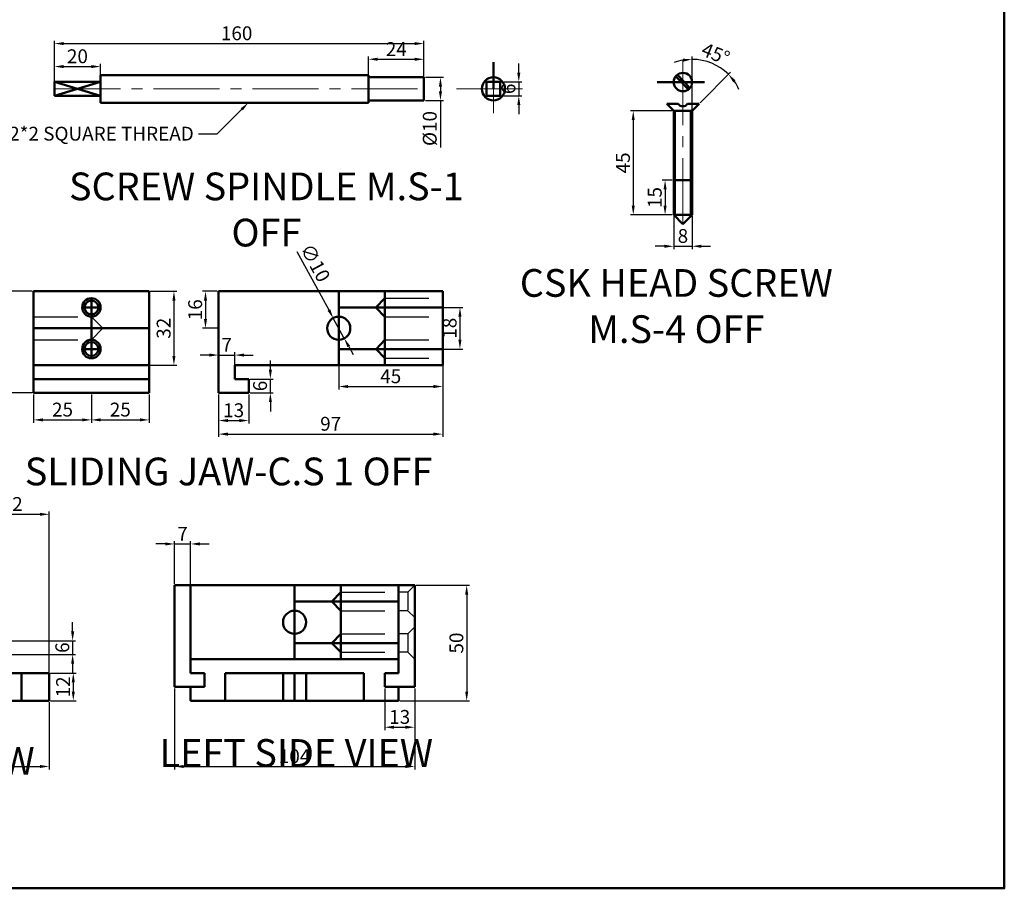
# Model space of a CAD drawing. Units: millimetres. Extents: x -1209 to -333, y 66 to 707.
# Tile 3 of 4: x -759 to -333, y 66 to 442. Entities that reach past the tile are written whole.
import ezdxf
from ezdxf import colors
from ezdxf.entities.mleader import LeaderData, LeaderLine
from ezdxf.math import Vec2, Vec3

# ---------------------------------------------------------------- set-up
doc = ezdxf.new("R2010")
doc.units = ezdxf.units.MM
doc.header["$LTSCALE"] = 1.5
doc.linetypes.add('CENTER2', pattern=[28.575, 19.05, -3.175, 3.175, -3.175])
doc.linetypes.add('DASHED', pattern=[19.05, 12.7, -6.35])
for name, color, linetype, lineweight in [('M-CNTR', 1, 'CENTER2', 18), ('M-DIMS', 2, 'Continuous', 25), ('M-HIDN', 4, 'DASHED', 25), ('M-OUTL', 7, 'Continuous', 50), ('M-TEXT', 3, 'Continuous', 25), ('M-TTLB', 7, 'Continuous', 50)]:
    doc.layers.add(name, color=color, linetype=linetype, lineweight=lineweight)
doc.styles.get("Standard").update_dxf_attribs({"font": 'arial.ttf'})
doc.dimstyles.new('ISO-25', dxfattribs={"dimtxt": 6, "dimasz": 4, "dimexe": 1.25, "dimexo": 0.625, "dimtad": 1, "dimdec": 0, "dimtxsty": 'Standard', "dimcen": 2.5, "dimadec": 0, "dimazin": 0, "dimtfac": 1, "dimtdec": 0, "dimtmove": 0, "dimatfit": 3, "dimfxl": 1, "dimarcsym": 0})

# ---------------------------------------------------------------- blocks, each defined once
blk = doc.blocks.new('*D24')
at = {"layer": 'Defpoints', "color": 0, "transparency": 16777216}
for p in [(-583.75, 431.73), (-743.75, 412.13), (-583.75, 412.13)]:
    blk.add_point(p, dxfattribs=at)
at = {"layer": 'M-DIMS', "color": 0, "lineweight": -2, "transparency": 16777216}
for p, q in [((-743.75, 412.76), (-743.75, 432.98)), ((-739.75, 431.73), (-587.75, 431.73)), ((-583.75, 412.76), (-583.75, 432.98))]:
    blk.add_line(p, q, dxfattribs=at)
at = {"layer": 'M-DIMS', "color": 0, "transparency": 16777216}
for points in [[(-739.75, 432.4), (-739.75, 431.07), (-743.75, 431.73)], [(-587.75, 432.4), (-587.75, 431.07), (-583.75, 431.73)]]:
    blk.add_solid(points, dxfattribs=at)
at = {"layer": 'M-DIMS', "color": 0, "transparency": 16777216, "insert": (-664.84, 435.42), "char_height": 6, "attachment_point": 5}
blk.add_mtext('160', dxfattribs=at)
blk = doc.blocks.new('*D25')
at = {"layer": 'Defpoints', "color": 0, "transparency": 16777216}
for p in [(-723.75, 421.78), (-743.75, 415.13), (-723.75, 415.13)]:
    blk.add_point(p, dxfattribs=at)
at = {"layer": 'M-DIMS', "color": 0, "lineweight": -2, "transparency": 16777216}
for p, q in [((-743.75, 415.76), (-743.75, 423.03)), ((-723.75, 415.76), (-723.75, 423.03)), ((-739.75, 421.78), (-727.75, 421.78))]:
    blk.add_line(p, q, dxfattribs=at)
at = {"layer": 'M-DIMS', "color": 0, "transparency": 16777216}
for points in [[(-739.75, 422.45), (-739.75, 421.11), (-743.75, 421.78)], [(-727.75, 422.45), (-727.75, 421.11), (-723.75, 421.78)]]:
    blk.add_solid(points, dxfattribs=at)
at = {"layer": 'M-DIMS', "color": 0, "transparency": 16777216, "insert": (-733.75, 425.47), "char_height": 6, "attachment_point": 5}
blk.add_mtext('20', dxfattribs=at)
blk = doc.blocks.new('*D26')
at = {"layer": 'Defpoints', "color": 0, "transparency": 16777216}
for p in [(-583.75, 424.94), (-607.75, 417.13), (-583.75, 417.13)]:
    blk.add_point(p, dxfattribs=at)
at = {"layer": 'M-DIMS', "color": 0, "lineweight": -2, "transparency": 16777216}
for p, q in [((-607.75, 417.76), (-607.75, 426.19)), ((-603.75, 424.94), (-587.75, 424.94)), ((-583.75, 417.76), (-583.75, 426.19))]:
    blk.add_line(p, q, dxfattribs=at)
at = {"layer": 'M-DIMS', "color": 0, "transparency": 16777216}
for points in [[(-603.75, 425.61), (-603.75, 424.28), (-607.75, 424.94)], [(-587.75, 425.61), (-587.75, 424.28), (-583.75, 424.94)]]:
    blk.add_solid(points, dxfattribs=at)
at = {"layer": 'M-DIMS', "color": 0, "transparency": 16777216, "insert": (-595.75, 428.58), "char_height": 6, "attachment_point": 5}
blk.add_mtext('24', dxfattribs=at)
blk = doc.blocks.new('*D27')
at = {"layer": 'Defpoints', "color": 0, "transparency": 16777216}
for p in [(-583.75, 417.13), (-583.75, 407.13), (-576.61, 407.13)]:
    blk.add_point(p, dxfattribs=at)
at = {"layer": 'M-DIMS', "color": 0, "lineweight": -2, "transparency": 16777216}
for p, q in [((-583.12, 417.13), (-575.36, 417.13)), ((-576.61, 413.13), (-576.61, 411.13)), ((-583.12, 407.13), (-575.36, 407.13)), ((-576.61, 407.13), (-576.61, 386.78))]:
    blk.add_line(p, q, dxfattribs=at)
at = {"layer": 'M-DIMS', "color": 0, "transparency": 16777216}
for points in [[(-577.28, 413.13), (-575.94, 413.13), (-576.61, 417.13)], [(-577.28, 411.13), (-575.94, 411.13), (-576.61, 407.13)]]:
    blk.add_solid(points, dxfattribs=at)
at = {"layer": 'M-DIMS', "color": 0, "transparency": 16777216, "insert": (-580.47, 394.96), "char_height": 6, "attachment_point": 5, "rotation": 90}
blk.add_mtext('%%C10', dxfattribs=at)
blk = doc.blocks.new('*D28')
at = {"layer": 'Defpoints', "color": 0, "transparency": 16777216}
for p in [(-550.71, 415.13), (-550.71, 409.13), (-542.7, 409.13)]:
    blk.add_point(p, dxfattribs=at)
at = {"layer": 'M-DIMS', "color": 0, "lineweight": -2, "transparency": 16777216}
for p, q in [((-542.7, 419.13), (-542.7, 423.13)), ((-550.08, 415.13), (-541.45, 415.13)), ((-542.7, 415.13), (-542.7, 409.13)), ((-550.08, 409.13), (-541.45, 409.13)), ((-542.7, 405.13), (-542.7, 401.13))]:
    blk.add_line(p, q, dxfattribs=at)
at = {"layer": 'M-DIMS', "color": 0, "transparency": 16777216}
for points in [[(-543.37, 419.13), (-542.03, 419.13), (-542.7, 415.13)], [(-543.37, 405.13), (-542.03, 405.13), (-542.7, 409.13)]]:
    blk.add_solid(points, dxfattribs=at)
at = {"layer": 'M-DIMS', "color": 0, "transparency": 16777216, "insert": (-546.39, 412.13), "char_height": 6, "attachment_point": 5, "rotation": 90}
blk.add_mtext('6', dxfattribs=at)
blk = doc.blocks.new('*D38')
at = {"layer": 'Defpoints', "color": 0, "transparency": 16777216}
for p in [(-575.63, 317.49), (-575.63, 299.49), (-568.17, 299.49)]:
    blk.add_point(p, dxfattribs=at)
at = {"layer": 'M-DIMS', "color": 0, "lineweight": -2, "transparency": 16777216}
for p, q in [((-575.01, 317.49), (-566.92, 317.49)), ((-568.17, 313.49), (-568.17, 303.49)), ((-575.01, 299.49), (-566.92, 299.49))]:
    blk.add_line(p, q, dxfattribs=at)
at = {"layer": 'M-DIMS', "color": 0, "transparency": 16777216}
for points in [[(-568.84, 313.49), (-567.51, 313.49), (-568.17, 317.49)], [(-568.84, 303.49), (-567.51, 303.49), (-568.17, 299.49)]]:
    blk.add_solid(points, dxfattribs=at)
at = {"layer": 'M-DIMS', "color": 0, "transparency": 16777216, "insert": (-571.86, 308.49), "char_height": 6, "attachment_point": 5, "rotation": 90}
blk.add_mtext('18', dxfattribs=at)
blk = doc.blocks.new('*D39')
at = {"layer": 'Defpoints', "color": 0, "transparency": 16777216}
for p in [(-620.63, 324.49), (-575.63, 324.49), (-575.63, 283.26)]:
    blk.add_point(p, dxfattribs=at)
at = {"layer": 'M-DIMS', "color": 0, "lineweight": -2, "transparency": 16777216}
for p, q in [((-620.63, 323.86), (-620.63, 282.01)), ((-575.63, 323.86), (-575.63, 282.01)), ((-616.63, 283.26), (-579.63, 283.26))]:
    blk.add_line(p, q, dxfattribs=at)
at = {"layer": 'M-DIMS', "color": 0, "transparency": 16777216}
for points in [[(-616.63, 283.92), (-616.63, 282.59), (-620.63, 283.26)], [(-579.63, 283.92), (-579.63, 282.59), (-575.63, 283.26)]]:
    blk.add_solid(points, dxfattribs=at)
at = {"layer": 'M-DIMS', "color": 0, "transparency": 16777216, "insert": (-598.13, 286.93), "char_height": 6, "attachment_point": 5}
blk.add_mtext('45', dxfattribs=at)
blk = doc.blocks.new('*D40')
at = {"layer": 'Defpoints', "color": 0, "transparency": 16777216}
for p in [(-752.7, 324.49), (-772.81, 280.49), (-752.7, 280.49)]:
    blk.add_point(p, dxfattribs=at)
at = {"layer": 'M-DIMS', "color": 0, "lineweight": -2, "transparency": 16777216}
for p, q in [((-753.33, 324.49), (-774.06, 324.49)), ((-772.81, 320.49), (-772.81, 284.49)), ((-753.33, 280.49), (-774.06, 280.49))]:
    blk.add_line(p, q, dxfattribs=at)
at = {"layer": 'M-DIMS', "color": 0, "transparency": 16777216}
for points in [[(-773.47, 320.49), (-772.14, 320.49), (-772.81, 324.49)], [(-773.47, 284.49), (-772.14, 284.49), (-772.81, 280.49)]]:
    blk.add_solid(points, dxfattribs=at)
at = {"layer": 'M-DIMS', "color": 0, "transparency": 16777216, "insert": (-776.43, 302.49), "char_height": 6, "attachment_point": 5, "rotation": 90}
blk.add_mtext('44', dxfattribs=at)
blk = doc.blocks.new('*D41')
at = {"layer": 'Defpoints', "color": 0, "transparency": 16777216}
for p in [(-702.7, 324.49), (-702.7, 292.49), (-691.98, 292.49)]:
    blk.add_point(p, dxfattribs=at)
at = {"layer": 'M-DIMS', "color": 0, "lineweight": -2, "transparency": 16777216}
for p, q in [((-702.08, 324.49), (-690.73, 324.49)), ((-691.98, 320.49), (-691.98, 296.49)), ((-702.08, 292.49), (-690.73, 292.49))]:
    blk.add_line(p, q, dxfattribs=at)
at = {"layer": 'M-DIMS', "color": 0, "transparency": 16777216}
for points in [[(-692.65, 320.49), (-691.32, 320.49), (-691.98, 324.49)], [(-692.65, 296.49), (-691.32, 296.49), (-691.98, 292.49)]]:
    blk.add_solid(points, dxfattribs=at)
at = {"layer": 'M-DIMS', "color": 0, "transparency": 16777216, "insert": (-695.67, 308.49), "char_height": 6, "attachment_point": 5, "rotation": 90}
blk.add_mtext('32', dxfattribs=at)
blk = doc.blocks.new('*D42')
at = {"layer": 'Defpoints', "color": 0, "transparency": 16777216}
for p in [(-752.7, 280.49), (-727.7, 280.49), (-727.7, 268.81)]:
    blk.add_point(p, dxfattribs=at)
at = {"layer": 'M-DIMS', "color": 0, "lineweight": -2, "transparency": 16777216}
for p, q in [((-752.7, 279.86), (-752.7, 267.56)), ((-727.7, 279.86), (-727.7, 267.56)), ((-748.7, 268.81), (-731.7, 268.81))]:
    blk.add_line(p, q, dxfattribs=at)
at = {"layer": 'M-DIMS', "color": 0, "transparency": 16777216}
for points in [[(-748.7, 269.48), (-748.7, 268.15), (-752.7, 268.81)], [(-731.7, 269.48), (-731.7, 268.15), (-727.7, 268.81)]]:
    blk.add_solid(points, dxfattribs=at)
at = {"layer": 'M-DIMS', "color": 0, "transparency": 16777216, "insert": (-740.2, 272.5), "char_height": 6, "attachment_point": 5}
blk.add_mtext('25', dxfattribs=at)
blk = doc.blocks.new('*D43')
at = {"layer": 'Defpoints', "color": 0, "transparency": 16777216}
for p in [(-727.7, 280.49), (-702.7, 280.49), (-702.7, 268.81)]:
    blk.add_point(p, dxfattribs=at)
at = {"layer": 'M-DIMS', "color": 0, "lineweight": -2, "transparency": 16777216}
for p, q in [((-727.7, 279.86), (-727.7, 267.56)), ((-702.7, 279.86), (-702.7, 267.56)), ((-723.7, 268.81), (-706.7, 268.81))]:
    blk.add_line(p, q, dxfattribs=at)
at = {"layer": 'M-DIMS', "color": 0, "transparency": 16777216}
for points in [[(-723.7, 269.48), (-723.7, 268.15), (-727.7, 268.81)], [(-706.7, 269.48), (-706.7, 268.15), (-702.7, 268.81)]]:
    blk.add_solid(points, dxfattribs=at)
at = {"layer": 'M-DIMS', "color": 0, "transparency": 16777216, "insert": (-715.2, 272.5), "char_height": 6, "attachment_point": 5}
blk.add_mtext('25', dxfattribs=at)
blk = doc.blocks.new('*D44')
at = {"layer": 'Defpoints', "color": 0, "transparency": 16777216}
for p in [(-672.63, 324.49), (-678.32, 308.49), (-672.63, 308.49)]:
    blk.add_point(p, dxfattribs=at)
at = {"layer": 'M-DIMS', "color": 0, "lineweight": -2, "transparency": 16777216}
for p, q in [((-673.26, 324.49), (-679.57, 324.49)), ((-678.32, 320.49), (-678.32, 312.49)), ((-673.26, 308.49), (-679.57, 308.49))]:
    blk.add_line(p, q, dxfattribs=at)
at = {"layer": 'M-DIMS', "color": 0, "transparency": 16777216}
for points in [[(-678.99, 320.49), (-677.66, 320.49), (-678.32, 324.49)], [(-678.99, 312.49), (-677.66, 312.49), (-678.32, 308.49)]]:
    blk.add_solid(points, dxfattribs=at)
at = {"layer": 'M-DIMS', "color": 0, "transparency": 16777216, "insert": (-682.01, 316.49), "char_height": 6, "attachment_point": 5, "rotation": 90}
blk.add_mtext('16', dxfattribs=at)
blk = doc.blocks.new('*D45')
at = {"layer": 'Defpoints', "color": 0, "transparency": 16777216}
for p in [(-575.63, 292.49), (-672.63, 280.49), (-575.63, 262.66)]:
    blk.add_point(p, dxfattribs=at)
at = {"layer": 'M-DIMS', "color": 0, "lineweight": -2, "transparency": 16777216}
for p, q in [((-575.63, 291.86), (-575.63, 261.41)), ((-672.63, 279.86), (-672.63, 261.41)), ((-668.63, 262.66), (-579.63, 262.66))]:
    blk.add_line(p, q, dxfattribs=at)
at = {"layer": 'M-DIMS', "color": 0, "transparency": 16777216}
for points in [[(-668.63, 263.33), (-668.63, 261.99), (-672.63, 262.66)], [(-579.63, 263.33), (-579.63, 261.99), (-575.63, 262.66)]]:
    blk.add_solid(points, dxfattribs=at)
at = {"layer": 'M-DIMS', "color": 0, "transparency": 16777216, "insert": (-624.13, 266.35), "char_height": 6, "attachment_point": 5}
blk.add_mtext('97', dxfattribs=at)
blk = doc.blocks.new('*D46')
at = {"layer": 'Defpoints', "color": 0, "transparency": 16777216}
for p in [(-672.63, 280.49), (-659.63, 280.49), (-659.63, 268.52)]:
    blk.add_point(p, dxfattribs=at)
at = {"layer": 'M-DIMS', "color": 0, "lineweight": -2, "transparency": 16777216}
for p, q in [((-672.63, 279.86), (-672.63, 267.27)), ((-659.63, 279.86), (-659.63, 267.27)), ((-668.63, 268.52), (-663.63, 268.52))]:
    blk.add_line(p, q, dxfattribs=at)
at = {"layer": 'M-DIMS', "color": 0, "transparency": 16777216}
for points in [[(-668.63, 269.19), (-668.63, 267.86), (-672.63, 268.52)], [(-663.63, 269.19), (-663.63, 267.86), (-659.63, 268.52)]]:
    blk.add_solid(points, dxfattribs=at)
at = {"layer": 'M-DIMS', "color": 0, "transparency": 16777216, "insert": (-666.13, 272.21), "char_height": 6, "attachment_point": 5}
blk.add_mtext('13', dxfattribs=at)
blk = doc.blocks.new('*D47')
at = {"layer": 'Defpoints', "color": 0, "transparency": 16777216}
for p in [(-665.63, 296.87), (-672.63, 287.82), (-665.63, 287.82)]:
    blk.add_point(p, dxfattribs=at)
at = {"layer": 'M-DIMS', "color": 0, "lineweight": -2, "transparency": 16777216}
for p, q in [((-676.63, 296.87), (-680.63, 296.87)), ((-672.63, 288.44), (-672.63, 298.12)), ((-672.63, 296.87), (-665.63, 296.87)), ((-665.63, 288.44), (-665.63, 298.12)), ((-661.63, 296.87), (-657.63, 296.87))]:
    blk.add_line(p, q, dxfattribs=at)
at = {"layer": 'M-DIMS', "color": 0, "transparency": 16777216}
for points in [[(-676.63, 297.54), (-676.63, 296.21), (-672.63, 296.87)], [(-661.63, 297.54), (-661.63, 296.21), (-665.63, 296.87)]]:
    blk.add_solid(points, dxfattribs=at)
at = {"layer": 'M-DIMS', "color": 0, "transparency": 16777216, "insert": (-669.13, 300.5), "char_height": 6, "attachment_point": 5}
blk.add_mtext('7', dxfattribs=at)
blk = doc.blocks.new('*D48')
at = {"layer": 'Defpoints', "color": 0, "transparency": 16777216}
for p in [(-659.63, 286.49), (-650.23, 286.49), (-659.63, 280.49)]:
    blk.add_point(p, dxfattribs=at)
at = {"layer": 'M-DIMS', "color": 0, "lineweight": -2, "transparency": 16777216}
for p, q in [((-650.23, 290.49), (-650.23, 294.49)), ((-659.01, 286.49), (-648.98, 286.49)), ((-650.23, 280.49), (-650.23, 286.49)), ((-659.01, 280.49), (-648.98, 280.49)), ((-650.23, 276.49), (-650.23, 272.49))]:
    blk.add_line(p, q, dxfattribs=at)
at = {"layer": 'M-DIMS', "color": 0, "transparency": 16777216}
for points in [[(-650.9, 290.49), (-649.56, 290.49), (-650.23, 286.49)], [(-650.9, 276.49), (-649.56, 276.49), (-650.23, 280.49)]]:
    blk.add_solid(points, dxfattribs=at)
at = {"layer": 'M-DIMS', "color": 0, "transparency": 16777216, "insert": (-653.92, 283.49), "char_height": 6, "attachment_point": 5, "rotation": 90}
blk.add_mtext('6', dxfattribs=at)
blk = doc.blocks.new('*D49')
at = {"layer": 'Defpoints', "color": 0, "transparency": 16777216}
for p in [(-475.63, 372.58), (-479.38, 357.58), (-475.63, 357.58)]:
    blk.add_point(p, dxfattribs=at)
at = {"layer": 'M-DIMS', "color": 0, "lineweight": -2, "transparency": 16777216}
for p, q in [((-476.25, 372.58), (-480.63, 372.58)), ((-479.38, 368.58), (-479.38, 361.58)), ((-476.25, 357.58), (-480.63, 357.58))]:
    blk.add_line(p, q, dxfattribs=at)
at = {"layer": 'M-DIMS', "color": 0, "transparency": 16777216}
for points in [[(-480.05, 368.58), (-478.71, 368.58), (-479.38, 372.58)], [(-480.05, 361.58), (-478.71, 361.58), (-479.38, 357.58)]]:
    blk.add_solid(points, dxfattribs=at)
at = {"layer": 'M-DIMS', "color": 0, "transparency": 16777216, "insert": (-483.07, 365.08), "char_height": 6, "attachment_point": 5, "rotation": 90}
blk.add_mtext('15', dxfattribs=at)
blk = doc.blocks.new('*D50')
at = {"layer": 'Defpoints', "color": 0, "transparency": 16777216}
for p in [(-475.66, 357.58), (-467.66, 357.58), (-467.66, 343.98)]:
    blk.add_point(p, dxfattribs=at)
at = {"layer": 'M-DIMS', "color": 0, "lineweight": -2, "transparency": 16777216}
for p, q in [((-475.66, 356.95), (-475.66, 342.73)), ((-467.66, 356.95), (-467.66, 342.73)), ((-479.66, 343.98), (-483.66, 343.98)), ((-475.66, 343.98), (-467.66, 343.98)), ((-463.66, 343.98), (-459.66, 343.98))]:
    blk.add_line(p, q, dxfattribs=at)
at = {"layer": 'M-DIMS', "color": 0, "transparency": 16777216}
for points in [[(-479.66, 344.65), (-479.66, 343.31), (-475.66, 343.98)], [(-463.66, 344.65), (-463.66, 343.31), (-467.66, 343.98)]]:
    blk.add_solid(points, dxfattribs=at)
at = {"layer": 'M-DIMS', "color": 0, "transparency": 16777216, "insert": (-471.66, 347.67), "char_height": 6, "attachment_point": 5}
blk.add_mtext('8', dxfattribs=at)
blk = doc.blocks.new('*D51')
at = {"layer": 'Defpoints', "color": 0, "transparency": 16777216}
for p in [(-475.66, 402.58), (-493.16, 357.58), (-475.63, 357.58)]:
    blk.add_point(p, dxfattribs=at)
at = {"layer": 'M-DIMS', "color": 0, "lineweight": -2, "transparency": 16777216}
for p, q in [((-476.28, 402.58), (-494.41, 402.58)), ((-493.16, 398.58), (-493.16, 361.58)), ((-476.25, 357.58), (-494.41, 357.58))]:
    blk.add_line(p, q, dxfattribs=at)
at = {"layer": 'M-DIMS', "color": 0, "transparency": 16777216}
for points in [[(-493.83, 398.58), (-492.5, 398.58), (-493.16, 402.58)], [(-493.83, 361.58), (-492.5, 361.58), (-493.16, 357.58)]]:
    blk.add_solid(points, dxfattribs=at)
at = {"layer": 'M-DIMS', "color": 0, "transparency": 16777216, "insert": (-496.84, 380.08), "char_height": 6, "attachment_point": 5, "rotation": 90}
blk.add_mtext('45', dxfattribs=at)
blk = doc.blocks.new('*D52')
at = {"layer": 'Defpoints', "color": 0, "transparency": 16777216}
for p in [(-456.56, 421.94), (-464.69, 405.58), (-467.66, 402.58), (-467.66, 402.58), (-467.66, 357.58)]:
    blk.add_point(p, dxfattribs=at)
at = {"layer": 'M-DIMS', "color": 0, "lineweight": -2, "transparency": 16777216}
for p, q in [((-467.66, 403.2), (-467.66, 426.15)), ((-464.25, 406.02), (-451.08, 419.32))]:
    blk.add_line(p, q, dxfattribs=at)
for start, end in [(100.2822, 110.5644), (45.2845, 90), (24.7201, 35.0023)]:
    blk.add_arc((-467.66, 402.58), 22.32, start, end, dxfattribs=at)
at = {"layer": 'M-DIMS', "color": 0, "transparency": 16777216}
for points in [[(-471.7, 425.2), (-471.58, 423.87), (-467.66, 424.9)], [(-449.89, 414.95), (-448.87, 415.81), (-451.96, 418.44)]]:
    blk.add_solid(points, dxfattribs=at)
at = {"layer": 'M-DIMS', "color": 0, "transparency": 16777216, "insert": (-457.77, 426.62), "char_height": 6, "attachment_point": 5, "rotation": 337.6422}
blk.add_mtext('45°', dxfattribs=at)
blk = doc.blocks.new('*D71')
at = {"layer": 'Defpoints', "color": 0, "ltscale": 0.4, "transparency": 16777216}
for p in [(-623.02, 312.88), (-618.24, 304.09)]:
    blk.add_point(p, dxfattribs=at)
at = {"layer": 'M-DIMS', "color": 0, "lineweight": -2, "ltscale": 0.4, "transparency": 16777216}
for p, q in [((-638.73, 341.76), (-624.93, 316.39)), ((-618.24, 304.09), (-623.02, 312.88)), ((-616.33, 300.58), (-614.42, 297.07))]:
    blk.add_line(p, q, dxfattribs=at)
at = {"layer": 'M-DIMS', "color": 0, "ltscale": 0.4, "transparency": 16777216}
for points in [[(-624.34, 316.71), (-625.52, 316.07), (-623.02, 312.88)], [(-615.74, 300.9), (-616.92, 300.26), (-618.24, 304.09)]]:
    blk.add_solid(points, dxfattribs=at)
at = {"layer": 'M-DIMS', "color": 0, "ltscale": 0.4, "transparency": 16777216, "insert": (-631.43, 336.42), "char_height": 6, "attachment_point": 5, "rotation": 298.5393}
blk.add_mtext('∅10', dxfattribs=at)
blk = doc.blocks.new('*D75')
at = {"layer": 'Defpoints', "color": 0, "ltscale": 0.4, "transparency": 16777216}
for p in [(-770.99, 173.2), (-770.99, 167.2), (-735.83, 167.2)]:
    blk.add_point(p, dxfattribs=at)
at = {"layer": 'M-DIMS', "color": 0, "lineweight": -2, "ltscale": 0.4, "transparency": 16777216}
for p, q in [((-735.83, 177.2), (-735.83, 181.2)), ((-770.37, 173.2), (-734.58, 173.2)), ((-735.83, 173.2), (-735.83, 167.2)), ((-770.37, 167.2), (-734.58, 167.2)), ((-735.83, 163.2), (-735.83, 159.2))]:
    blk.add_line(p, q, dxfattribs=at)
at = {"layer": 'M-DIMS', "color": 0, "ltscale": 0.4, "transparency": 16777216}
for points in [[(-736.5, 177.2), (-735.16, 177.2), (-735.83, 173.2)], [(-736.5, 163.2), (-735.16, 163.2), (-735.83, 167.2)]]:
    blk.add_solid(points, dxfattribs=at)
at = {"layer": 'M-DIMS', "color": 0, "ltscale": 0.4, "transparency": 16777216, "insert": (-739.52, 170.2), "char_height": 6, "attachment_point": 5, "rotation": 90}
blk.add_mtext('6', dxfattribs=at)
blk = doc.blocks.new('*D76')
at = {"layer": 'Defpoints', "color": 0, "ltscale": 0.4, "transparency": 16777216}
for p in [(-745.99, 159.2), (-745.99, 147.2), (-735.55, 147.2)]:
    blk.add_point(p, dxfattribs=at)
at = {"layer": 'M-DIMS', "color": 0, "lineweight": -2, "ltscale": 0.4, "transparency": 16777216}
for p, q in [((-745.37, 159.2), (-734.3, 159.2)), ((-735.55, 155.2), (-735.55, 151.2)), ((-745.37, 147.2), (-734.3, 147.2))]:
    blk.add_line(p, q, dxfattribs=at)
at = {"layer": 'M-DIMS', "color": 0, "ltscale": 0.4, "transparency": 16777216}
for points in [[(-736.22, 155.2), (-734.88, 155.2), (-735.55, 159.2)], [(-736.22, 151.2), (-734.88, 151.2), (-735.55, 147.2)]]:
    blk.add_solid(points, dxfattribs=at)
at = {"layer": 'M-DIMS', "color": 0, "ltscale": 0.4, "transparency": 16777216, "insert": (-739.19, 153.2), "char_height": 6, "attachment_point": 5, "rotation": 90}
blk.add_mtext('12', dxfattribs=at)
blk = doc.blocks.new('*D77')
at = {"layer": 'Defpoints', "color": 0, "ltscale": 0.4, "transparency": 16777216}
for p in [(-684.76, 215.1), (-691.76, 197.2), (-684.76, 197.2)]:
    blk.add_point(p, dxfattribs=at)
at = {"layer": 'M-DIMS', "color": 0, "lineweight": -2, "ltscale": 0.4, "transparency": 16777216}
for p, q in [((-695.76, 215.1), (-699.76, 215.1)), ((-691.76, 197.83), (-691.76, 216.35)), ((-691.76, 215.1), (-684.76, 215.1)), ((-684.76, 197.83), (-684.76, 216.35)), ((-680.76, 215.1), (-676.76, 215.1))]:
    blk.add_line(p, q, dxfattribs=at)
at = {"layer": 'M-DIMS', "color": 0, "ltscale": 0.4, "transparency": 16777216}
for points in [[(-695.76, 215.76), (-695.76, 214.43), (-691.76, 215.1)], [(-680.76, 215.76), (-680.76, 214.43), (-684.76, 215.1)]]:
    blk.add_solid(points, dxfattribs=at)
at = {"layer": 'M-DIMS', "color": 0, "ltscale": 0.4, "transparency": 16777216, "insert": (-688.26, 218.72), "char_height": 6, "attachment_point": 5}
blk.add_mtext('7', dxfattribs=at)
blk = doc.blocks.new('*D78')
at = {"layer": 'Defpoints', "color": 0, "ltscale": 0.4, "transparency": 16777216}
for p in [(-600.76, 153.2), (-587.76, 153.2), (-587.76, 135.75)]:
    blk.add_point(p, dxfattribs=at)
at = {"layer": 'M-DIMS', "color": 0, "lineweight": -2, "ltscale": 0.4, "transparency": 16777216}
for p, q in [((-600.76, 152.58), (-600.76, 134.5)), ((-587.76, 152.58), (-587.76, 134.5)), ((-596.76, 135.75), (-591.76, 135.75))]:
    blk.add_line(p, q, dxfattribs=at)
at = {"layer": 'M-DIMS', "color": 0, "ltscale": 0.4, "transparency": 16777216}
for points in [[(-596.76, 136.41), (-596.76, 135.08), (-600.76, 135.75)], [(-591.76, 136.41), (-591.76, 135.08), (-587.76, 135.75)]]:
    blk.add_solid(points, dxfattribs=at)
at = {"layer": 'M-DIMS', "color": 0, "ltscale": 0.4, "transparency": 16777216, "insert": (-594.26, 139.44), "char_height": 6, "attachment_point": 5}
blk.add_mtext('13', dxfattribs=at)
blk = doc.blocks.new('*D82')
at = {"layer": 'Defpoints', "color": 0, "ltscale": 1.5, "transparency": 16777216}
for p in [(-745.99, 227.93), (-777.99, 199.2), (-745.99, 147.2)]:
    blk.add_point(p, dxfattribs=at)
at = {"layer": 'M-DIMS', "color": 0, "lineweight": -2, "ltscale": 1.5, "transparency": 16777216}
for p, q in [((-777.99, 199.83), (-777.99, 229.18)), ((-773.99, 227.93), (-749.99, 227.93)), ((-745.99, 147.83), (-745.99, 229.18))]:
    blk.add_line(p, q, dxfattribs=at)
at = {"layer": 'M-DIMS', "color": 0, "ltscale": 1.5, "transparency": 16777216}
for points in [[(-773.99, 228.6), (-773.99, 227.26), (-777.99, 227.93)], [(-749.99, 228.6), (-749.99, 227.26), (-745.99, 227.93)]]:
    blk.add_solid(points, dxfattribs=at)
at = {"layer": 'M-DIMS', "color": 0, "ltscale": 1.5, "transparency": 16777216, "insert": (-761.99, 231.62), "char_height": 6, "attachment_point": 5}
blk.add_mtext('32', dxfattribs=at)
blk = doc.blocks.new('*D83')
at = {"layer": 'Defpoints', "color": 0, "ltscale": 1.5, "transparency": 16777216}
for p in [(-960.99, 147.2), (-745.99, 147.2), (-745.99, 118.76)]:
    blk.add_point(p, dxfattribs=at)
at = {"layer": 'M-DIMS', "color": 0, "lineweight": -2, "ltscale": 1.5, "transparency": 16777216}
for p, q in [((-960.99, 146.58), (-960.99, 117.51)), ((-745.99, 146.58), (-745.99, 117.51)), ((-956.99, 118.76), (-749.99, 118.76))]:
    blk.add_line(p, q, dxfattribs=at)
at = {"layer": 'M-DIMS', "color": 0, "ltscale": 1.5, "transparency": 16777216}
for points in [[(-956.99, 119.42), (-956.99, 118.09), (-960.99, 118.76)], [(-749.99, 119.42), (-749.99, 118.09), (-745.99, 118.76)]]:
    blk.add_solid(points, dxfattribs=at)
at = {"layer": 'M-DIMS', "color": 0, "ltscale": 1.5, "transparency": 16777216, "insert": (-853.49, 122.44), "char_height": 6, "attachment_point": 5}
blk.add_mtext('215', dxfattribs=at)
blk = doc.blocks.new('*D85')
at = {"layer": 'Defpoints', "color": 0, "ltscale": 1.5, "transparency": 16777216}
for p in [(-691.76, 153.2), (-587.76, 153.2), (-587.76, 118.76)]:
    blk.add_point(p, dxfattribs=at)
at = {"layer": 'M-DIMS', "color": 0, "lineweight": -2, "ltscale": 1.5, "transparency": 16777216}
for p, q in [((-691.76, 152.58), (-691.76, 117.51)), ((-587.76, 152.58), (-587.76, 117.51)), ((-687.76, 118.76), (-591.76, 118.76))]:
    blk.add_line(p, q, dxfattribs=at)
at = {"layer": 'M-DIMS', "color": 0, "ltscale": 1.5, "transparency": 16777216}
for points in [[(-687.76, 119.42), (-687.76, 118.09), (-691.76, 118.76)], [(-591.76, 119.42), (-591.76, 118.09), (-587.76, 118.76)]]:
    blk.add_solid(points, dxfattribs=at)
at = {"layer": 'M-DIMS', "color": 0, "ltscale": 1.5, "transparency": 16777216, "insert": (-639.76, 122.44), "char_height": 6, "attachment_point": 5}
blk.add_mtext('104', dxfattribs=at)
blk = doc.blocks.new('*D86')
at = {"layer": 'Defpoints', "color": 0, "ltscale": 1.5, "transparency": 16777216}
for p in [(-587.76, 197.2), (-594.76, 147.2), (-565.26, 147.2)]:
    blk.add_point(p, dxfattribs=at)
at = {"layer": 'M-DIMS', "color": 0, "lineweight": -2, "ltscale": 1.5, "transparency": 16777216}
for p, q in [((-587.14, 197.2), (-564.01, 197.2)), ((-565.26, 193.2), (-565.26, 151.2)), ((-594.14, 147.2), (-564.01, 147.2))]:
    blk.add_line(p, q, dxfattribs=at)
at = {"layer": 'M-DIMS', "color": 0, "ltscale": 1.5, "transparency": 16777216}
for points in [[(-565.93, 193.2), (-564.59, 193.2), (-565.26, 197.2)], [(-565.93, 151.2), (-564.59, 151.2), (-565.26, 147.2)]]:
    blk.add_solid(points, dxfattribs=at)
at = {"layer": 'M-DIMS', "color": 0, "ltscale": 1.5, "transparency": 16777216, "insert": (-568.95, 172.2), "char_height": 6, "attachment_point": 5, "rotation": 90}
blk.add_mtext('50', dxfattribs=at)

msp = doc.modelspace()

# ---------------------------------------------------------------- linework, layer by layer
at = {"layer": 'M-CNTR'}
for p, q in [((-553.71, 423.75), (-553.71, 401.56)), ((-471.66, 353.6), (-471.66, 424.53)), ((-743.75, 412.13), (-583.75, 412.13)), ((-569.6, 412.13), (-537.82, 412.13))]:
    msp.add_line(p, q, dxfattribs=at)
at = {"layer": 'M-HIDN'}
for p, q in [((-600.63, 321.49), (-575.63, 321.49)), ((-752.7, 313.49), (-727.7, 313.49)), ((-727.7, 313.49), (-722.7, 308.47)), ((-600.63, 313.49), (-575.63, 313.49)), ((-727.7, 303.49), (-722.69, 308.49)), ((-752.7, 303.49), (-727.7, 303.49)), ((-600.63, 303.49), (-575.63, 303.49)), ((-600.63, 295.49), (-575.63, 295.49)), ((-619.76, 194.2), (-594.76, 194.2)), ((-619.76, 186.2), (-594.76, 186.2)), ((-619.76, 176.2), (-594.76, 176.2)), ((-619.76, 168.2), (-594.76, 168.2))]:
    msp.add_line(p, q, dxfattribs=at)
at = {"layer": 'M-HIDN', "ltscale": 0.4}
for p, q in [((-590.76, 194.2), (-587.76, 197.2)), ((-590.76, 194.2), (-594.76, 194.2)), ((-590.76, 194.2), (-590.76, 186.2)), ((-590.76, 186.2), (-594.76, 186.2)), ((-590.76, 186.2), (-587.76, 183.2)), ((-590.76, 176.2), (-587.76, 179.2)), ((-590.76, 176.2), (-594.76, 176.2)), ((-590.76, 176.2), (-590.76, 168.2)), ((-590.76, 168.2), (-594.76, 168.2)), ((-590.76, 168.2), (-587.76, 165.2))]:
    msp.add_line(p, q, dxfattribs=at)
at = {"layer": 'M-OUTL'}
for p, q in [((-553.71, 412.13), (-553.71, 423.75)), ((-723.75, 407.13), (-723.75, 418.13)), ((-723.75, 418.13), (-665.75, 418.13)), ((-607.75, 418.13), (-665.75, 418.13)), ((-607.75, 407.13), (-607.75, 418.13)), ((-474, 418.2), (-468.45, 412.43)), ((-723.75, 415.13), (-743.75, 415.13)), ((-743.75, 409.13), (-743.75, 415.13)), ((-743.75, 415.13), (-723.75, 409.13)), ((-743.75, 409.13), (-723.75, 415.13)), ((-583.75, 417.13), (-607.75, 417.13)), ((-583.75, 417.13), (-583.75, 407.13)), ((-482.74, 415.06), (-462.31, 415.06)), ((-474.68, 417.51), (-469.14, 411.74)), ((-723.75, 409.13), (-743.75, 409.13)), ((-723.75, 407.13), (-723.75, 406.13)), ((-723.75, 406.13), (-665.75, 406.13)), ((-607.75, 406.13), (-665.75, 406.13)), ((-583.75, 407.13), (-607.75, 407.13)), ((-607.75, 407.13), (-607.75, 406.13)), ((-475.66, 402.58), (-478.65, 405.58)), ((-473.67, 405.58), (-478.65, 405.58)), ((-464.69, 405.58), (-469.67, 405.58)), ((-467.66, 402.58), (-464.69, 405.58)), ((-475.66, 402.58), (-475.66, 357.58)), ((-467.66, 402.58), (-475.66, 402.58)), ((-475.16, 402.58), (-475.16, 357.58)), ((-468.16, 357.58), (-468.16, 402.58)), ((-467.66, 357.58), (-467.66, 402.58)), ((-475.63, 372.58), (-467.63, 372.58)), ((-475.66, 357.58), (-467.66, 357.58)), ((-471.66, 353.6), (-475.66, 357.58)), ((-467.66, 357.58), (-471.66, 353.6)), ((-702.7, 324.49), (-752.7, 324.49)), ((-752.7, 324.49), (-752.7, 280.49)), ((-702.7, 308.49), (-702.7, 324.49)), ((-575.63, 324.49), (-672.63, 324.49)), ((-672.63, 324.49), (-672.63, 280.49)), ((-620.63, 292.49), (-620.63, 324.49)), ((-600.63, 324.49), (-600.63, 292.49)), ((-575.63, 324.49), (-575.63, 292.49)), ((-727.7, 295.49), (-727.7, 321.49)), ((-604.57, 317.49), (-600.63, 321.49)), ((-731.7, 317.49), (-723.7, 317.49)), ((-620.63, 317.49), (-575.63, 317.49)), ((-600.63, 313.49), (-604.57, 317.49)), ((-752.7, 308.49), (-702.7, 308.49)), ((-702.7, 280.49), (-702.7, 308.49)), ((-604.47, 299.49), (-600.63, 303.49)), ((-731.7, 299.49), (-723.7, 299.49)), ((-620.63, 299.49), (-575.63, 299.49)), ((-600.63, 295.49), (-604.47, 299.49)), ((-702.7, 292.49), (-752.7, 292.49)), ((-575.63, 292.49), (-665.63, 292.49)), ((-665.63, 286.47), (-665.63, 292.49)), ((-752.7, 286.49), (-727.7, 286.49)), ((-727.7, 286.49), (-702.7, 286.49)), ((-665.63, 286.47), (-659.63, 286.47)), ((-659.63, 280.49), (-659.63, 286.49)), ((-752.7, 280.49), (-727.7, 280.49)), ((-727.7, 280.49), (-702.7, 280.49)), ((-672.63, 280.49), (-659.63, 280.49)), ((-587.76, 197.2), (-691.76, 197.2)), ((-691.76, 197.2), (-691.76, 153.2)), ((-639.76, 165.2), (-639.76, 197.2)), ((-619.76, 197.2), (-619.76, 165.2)), ((-594.76, 197.2), (-594.76, 165.2)), ((-587.76, 197.2), (-587.76, 153.2)), ((-623.7, 190.2), (-619.76, 194.2)), ((-639.76, 190.2), (-594.76, 190.2)), ((-619.76, 186.2), (-623.7, 190.2)), ((-623.6, 172.2), (-619.76, 176.2)), ((-639.76, 172.2), (-594.76, 172.2)), ((-619.76, 168.2), (-623.6, 172.2)), ((-594.76, 165.2), (-684.76, 165.2)), ((-684.76, 159.19), (-684.76, 165.2)), ((-594.76, 159.19), (-594.76, 165.2)), ((-684.76, 159.19), (-678.76, 159.19)), ((-678.76, 153.2), (-678.76, 159.2)), ((-600.76, 153.2), (-600.76, 159.2)), ((-594.76, 159.19), (-600.76, 159.19)), ((-691.76, 153.2), (-678.76, 153.2)), ((-587.76, 153.2), (-600.76, 153.2))]:
    msp.add_line(p, q, dxfattribs=at)
at = {"layer": 'M-OUTL', "ltscale": 0.4}
for p, q in [((-684.76, 165.2), (-684.76, 197.2)), ((-590.76, 197.2), (-594.76, 197.2)), ((-594.76, 197.2), (-594.76, 159.2)), ((-587.76, 197.2), (-590.76, 197.2)), ((-587.76, 153.2), (-587.76, 197.2)), ((-745.99, 159.2), (-770.99, 159.2)), ((-757.99, 147.2), (-757.99, 159.2)), ((-745.99, 147.2), (-745.99, 159.2)), ((-609.76, 159.2), (-669.76, 159.18)), ((-669.76, 159.18), (-669.76, 147.2)), ((-644.76, 159.19), (-644.76, 147.2)), ((-639.76, 159.19), (-639.76, 147.2)), ((-634.76, 159.19), (-634.76, 147.2)), ((-609.76, 147.2), (-609.76, 159.2)), ((-600.76, 159.2), (-600.76, 153.2)), ((-684.76, 153.2), (-684.76, 147.2)), ((-600.76, 153.2), (-587.76, 153.2)), ((-594.76, 147.2), (-594.76, 153.2)), ((-783.99, 147.2), (-745.99, 147.2)), ((-684.76, 147.2), (-594.76, 147.2)), ((-639.76, 147.2), (-609.76, 147.2))]:
    msp.add_line(p, q, dxfattribs=at)
at = {"layer": 'M-OUTL'}
msp.add_lwpolyline([(-556.71, 415.13), (-550.71, 415.13), (-550.71, 409.13), (-556.71, 409.13)], close=True, dxfattribs=at)
for centre, radius in [((-471.66, 415.06), 4), ((-553.71, 412.13), 5), ((-727.7, 317.49), 4), ((-620.63, 308.49), 5), ((-727.7, 299.49), 4), ((-639.76, 181.2), 5)]:
    msp.add_circle(centre, radius, dxfattribs=at)
at = {"layer": 'M-OUTL', "ltscale": 0.4}
for centre in [(-727.7, 317.49), (-727.7, 299.49)]:
    msp.add_circle(centre, 3, dxfattribs=at)
at = {"layer": 'M-OUTL'}
msp.add_arc((-471.67, 407.08), 2.5, 216.8582, 323.1418, dxfattribs=at)
at = {"layer": 'M-TTLB', "ltscale": 0.4}
msp.add_lwpolyline([(-1209.09, 706.73), (-332.54, 706.73), (-332.54, 66.01), (-1209.09, 66.01)], close=True, dxfattribs=at)

# ---------------------------------------------------------------- texts
at = {"layer": 'M-TEXT', "ltscale": 0.4, "char_height": 12, "attachment_point": 1}
for s, width, insert in [('\\pxqc;SCREW SPINDLE M.S-1 OFF', 194.7921, (-749.36, 375.9)), ('\\pxqc;CSK HEAD SCREW M.S-4 OFF', 177.8457, (-563.43, 334.1)), ('\\pxqc;SLIDING JAW-C.S 1 OFF', 196.4568, (-766.54, 252.49)), ('\\pxqc;LEFT SIDE VIEW', 177.8457, (-727.94, 130.6)), ('\\pxqc;SECTIONAL FRONT VIEW', 207.9769, (-949.26, 127.24))]:
    msp.add_mtext_dynamic_manual_height_columns(s, width=width, gutter_width=12.5, heights=[0], dxfattribs=dict(at, insert=insert))

# ---------------------------------------------------------------- dimensions: what is measured, and where the dimension line sits
at = {"layer": 'M-DIMS'}
for base, p1, p2, picture, middle in [((-583.75, 431.73), (-743.75, 412.13), (-583.75, 412.13), '*D24', (-664.84, 431.73)), ((-467.66, 343.98), (-475.66, 357.58), (-467.66, 357.58), '*D50', (-471.66, 343.98)), ((-575.63, 283.26), (-620.63, 324.49), (-575.63, 324.49), '*D39', (-598.13, 283.26)), ((-575.63, 262.66), (-672.63, 280.49), (-575.63, 292.49), '*D45', (-624.13, 262.66)), ((-659.63, 268.52), (-672.63, 280.49), (-659.63, 280.49), '*D46', (-666.13, 268.52))]:
    dim = msp.add_linear_dim(base=base, p1=p1, p2=p2, dimstyle='ISO-25', override={"dimclrd": 0, "dimclre": 0, "dimclrt": 0}, dxfattribs=at)
    dim.commit()
    dim.dimension.update_dxf_attribs({"geometry": picture, "text_midpoint": middle, "dimtype": 160})
for base, p1, p2, picture, middle in [((-583.75, 424.94), (-607.75, 417.13), (-583.75, 417.13), '*D26', (-595.75, 428.58)), ((-723.75, 421.78), (-743.75, 415.13), (-723.75, 415.13), '*D25', (-733.75, 425.47)), ((-665.63, 296.87), (-672.63, 287.82), (-665.63, 287.82), '*D47', (-669.13, 300.5)), ((-727.7, 268.81), (-752.7, 280.49), (-727.7, 280.49), '*D42', (-740.2, 272.5)), ((-702.7, 268.81), (-727.7, 280.49), (-702.7, 280.49), '*D43', (-715.2, 272.5))]:
    dim = msp.add_linear_dim(base=base, p1=p1, p2=p2, dimstyle='ISO-25', override={"dimclrd": 0, "dimclre": 0, "dimclrt": 0}, dxfattribs=at)
    dim.commit()
    dim.dimension.update_dxf_attribs({"geometry": picture, "text_midpoint": middle})
dim = msp.add_angular_dim_2l(base=(-456.56, 421.94), line1=((-467.66, 357.58), (-467.66, 402.58)), line2=((-467.66, 402.58), (-464.69, 405.58)), dimstyle='ISO-25', override={"dimclrd": 0, "dimclre": 0, "dimclrt": 0}, dxfattribs=at)
dim.commit()
dim.dimension.update_dxf_attribs({"geometry": '*D52', "text_midpoint": (-457.77, 426.62)})
for base, p1, p2, picture, middle in [((-542.7, 409.13), (-550.71, 415.13), (-550.71, 409.13), '*D28', (-546.39, 412.13)), ((-493.16, 357.58), (-475.66, 402.58), (-475.63, 357.58), '*D51', (-496.84, 380.08)), ((-479.38, 357.58), (-475.63, 372.58), (-475.63, 357.58), '*D49', (-483.07, 365.08)), ((-772.81, 280.49), (-752.7, 324.49), (-752.7, 280.49), '*D40', (-776.43, 302.49)), ((-568.17, 299.49), (-575.63, 317.49), (-575.63, 299.49), '*D38', (-571.86, 308.49))]:
    dim = msp.add_linear_dim(base=base, p1=p1, p2=p2, angle=90, dimstyle='ISO-25', override={"dimclrd": 0, "dimclre": 0, "dimclrt": 0}, dxfattribs=at)
    dim.commit()
    dim.dimension.update_dxf_attribs({"geometry": picture, "text_midpoint": middle})
dim = msp.add_linear_dim(base=(-576.61, 407.13), p1=(-583.75, 417.13), p2=(-583.75, 407.13), angle=90, text='%%C<>', dimstyle='ISO-25', override={"dimclrd": 0, "dimclre": 0, "dimclrt": 0}, dxfattribs=at)
dim.commit()
dim.dimension.update_dxf_attribs({"geometry": '*D27', "text_midpoint": (-580.47, 394.96)})
at = {"layer": 'M-DIMS', "ltscale": 0.4}
dim = msp.add_diameter_dim_2p(p1=(-618.24, 304.09), p2=(-623.02, 312.88), dimstyle='ISO-25', override={"dimclrd": 0, "dimclre": 0, "dimclrt": 0}, dxfattribs=at)
dim.commit()
dim.dimension.update_dxf_attribs({"geometry": '*D71', "text_midpoint": (-634.82, 334.58), "dimtype": 163})
at = {"layer": 'M-DIMS'}
for base, p1, p2, picture, middle in [((-691.98, 292.49), (-702.7, 324.49), (-702.7, 292.49), '*D41', (-691.98, 308.49)), ((-678.32, 308.49), (-672.63, 324.49), (-672.63, 308.49), '*D44', (-678.32, 316.49)), ((-650.23, 286.49), (-659.63, 280.49), (-659.63, 286.49), '*D48', (-650.23, 283.49))]:
    dim = msp.add_linear_dim(base=base, p1=p1, p2=p2, angle=90, dimstyle='ISO-25', override={"dimclrd": 0, "dimclre": 0, "dimclrt": 0}, dxfattribs=at)
    dim.commit()
    dim.dimension.update_dxf_attribs({"geometry": picture, "text_midpoint": middle, "dimtype": 160})
at = {"layer": 'M-DIMS', "ltscale": 1.5}
for base, p1, p2, picture, middle in [((-745.99, 227.93), (-777.99, 199.2), (-745.99, 147.2), '*D82', (-761.99, 231.62)), ((-587.76, 118.76), (-691.76, 153.2), (-587.76, 153.2), '*D85', (-639.76, 122.44)), ((-745.99, 118.76), (-960.99, 147.2), (-745.99, 147.2), '*D83', (-853.49, 122.44))]:
    dim = msp.add_linear_dim(base=base, p1=p1, p2=p2, dimstyle='ISO-25', override={"dimdec": 0, "dimlfac": 1, "dimrnd": 0, "dimzin": 0, "dimdsep": 46, "dimlunit": 2}, dxfattribs=at)
    dim.commit()
    dim.dimension.update_dxf_attribs({"geometry": picture, "text_midpoint": middle})
at = {"layer": 'M-DIMS', "ltscale": 0.4}
dim = msp.add_linear_dim(base=(-684.76, 215.1), p1=(-691.76, 197.2), p2=(-684.76, 197.2), dimstyle='ISO-25', override={"dimclrd": 0, "dimclre": 0, "dimclrt": 0}, dxfattribs=at)
dim.commit()
dim.dimension.update_dxf_attribs({"geometry": '*D77', "text_midpoint": (-688.26, 218.72)})
at = {"layer": 'M-DIMS', "ltscale": 1.5}
dim = msp.add_linear_dim(base=(-565.26, 147.2), p1=(-587.76, 197.2), p2=(-594.76, 147.2), angle=90, dimstyle='ISO-25', override={"dimdec": 0, "dimlfac": 1, "dimrnd": 0, "dimzin": 0, "dimdsep": 46, "dimlunit": 2}, dxfattribs=at)
dim.commit()
dim.dimension.update_dxf_attribs({"geometry": '*D86', "text_midpoint": (-568.95, 172.2)})
at = {"layer": 'M-DIMS', "ltscale": 0.4}
for base, p1, p2, picture, middle in [((-735.83, 167.2), (-770.99, 173.2), (-770.99, 167.2), '*D75', (-739.52, 170.2)), ((-735.55, 147.2), (-745.99, 159.2), (-745.99, 147.2), '*D76', (-739.19, 153.2))]:
    dim = msp.add_linear_dim(base=base, p1=p1, p2=p2, angle=90, dimstyle='ISO-25', override={"dimclrd": 0, "dimclre": 0, "dimclrt": 0}, dxfattribs=at)
    dim.commit()
    dim.dimension.update_dxf_attribs({"geometry": picture, "text_midpoint": middle})
dim = msp.add_linear_dim(base=(-587.76, 135.75), p1=(-600.76, 153.2), p2=(-587.76, 153.2), dimstyle='ISO-25', override={"dimclrd": 0, "dimclre": 0, "dimclrt": 0}, dxfattribs=at)
dim.commit()
dim.dimension.update_dxf_attribs({"geometry": '*D78', "text_midpoint": (-594.26, 135.75), "dimtype": 160})

# ---------------------------------------------------------------- leaders
ml = msp.add_multileader_mtext('Standard', dxfattribs=at)
ml.set_content('M12*2 SQUARE THREAD', color=256)
ml.set_leader_properties()
ml.build(insert=Vec2(0, 0))
ctx = ml.context
ctx.base_point, ctx.char_height, ctx.plane_origin = Vec3(-783.06, 392.49), 6, Vec3(-659.75, 406.13)
ctx.text_align_type = 2
notes = []
notes.append((ctx, [(0, (1, 1, 0), (-673.39, 392.49), (-1, 0), 8, [(0, [(-659.75, 406.13)], 0, [])])]))
ctx.mtext.insert, ctx.mtext.alignment, ctx.mtext.flow_direction = Vec3(-683.39, 395.73), 3, 5
for ctx, leaders in notes:
    for number, flags, end, landing, length, lines in leaders:
        leader = LeaderData()
        leader.index, (leader.has_last_leader_line, leader.has_dogleg_vector, leader.attachment_direction) = number, flags
        leader.last_leader_point, leader.dogleg_vector, leader.dogleg_length = Vec3(end), Vec3(landing), length
        for number, points, colour, breaks in lines:
            line = LeaderLine()
            line.index, line.vertices, line.color, line.breaks = number, Vec3.list(points), colors.encode_raw_color(colour), breaks
            leader.lines.append(line)
        ctx.leaders.append(leader)

doc.saveas('drawing.dxf')
